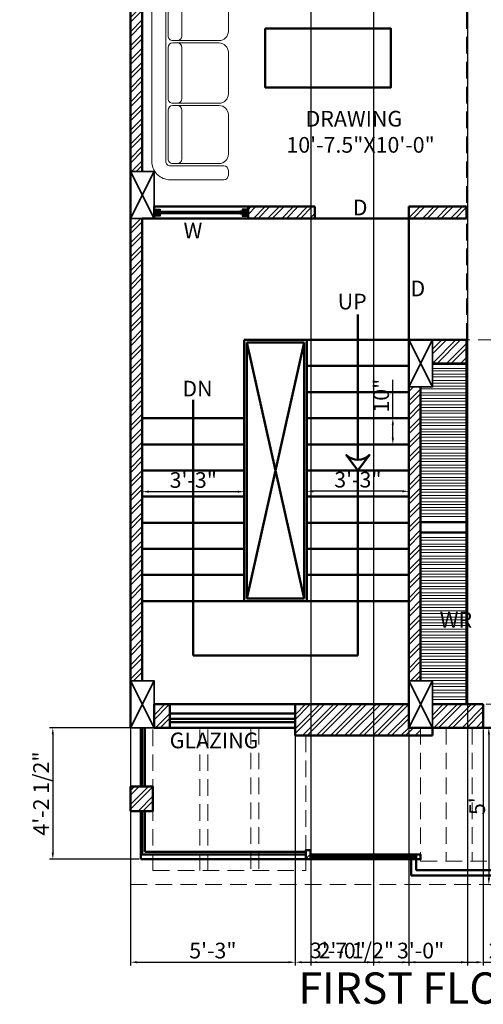
# Model space of a CAD drawing. Units: millimetres. Extents: x 67033 to 68301, y 155969 to 157209.
# Tile 10 of 17: x 67456 to 67633, y 156517 to 156894. Entities that reach past the tile are written whole.
import ezdxf

# ---------------------------------------------------------------- set-up
doc = ezdxf.new("R2010")
doc.units = ezdxf.units.MM
doc.linetypes.add('HIDDEN', pattern=[9.525, 6.35, -3.175])
for name, color, linetype, lineweight in [('A-ANNO-DIMS', 2, 'Continuous', 18), ('A-ANNO-TEXT', 7, 'Continuous', 18), ('A-AREA-IDEN', 3, 'Continuous', 18), ('A-COLS', 3, 'Continuous', 35), ('A-FLOR-OVHD', 1, 'HIDDEN', 18), ('A-FURN', 8, 'Continuous', 18), ('A-GLAZ', 4, 'Continuous', 25), ('A-WALL', 7, 'Continuous', 50), ('A-WALL-PATT', 8, 'Continuous', 13)]:
    doc.layers.add(name, color=color, linetype=linetype, lineweight=lineweight)
doc.styles.get("Standard").update_dxf_attribs({"font": 'arial.ttf'})
doc.dimstyles.new('ISO-25', dxfattribs={"dimtxt": 6, "dimasz": 2.5, "dimexe": 1.25, "dimexo": 0.625, "dimtad": 1, "dimdec": 0, "dimlunit": 3, "dimtxsty": 'Standard', "dimcen": 2.5, "dimadec": 0, "dimazin": 0, "dimtfac": 1, "dimtdec": 0, "dimtmove": 0, "dimatfit": 3, "dimfxl": 1, "dimarcsym": 0})
pattern_1 = [(45, (429.8785, 0), (-2.69407684, 2.69407684), []), (45, (431.6745, 0), (-2.69407684, 2.69407684), [])]

# ---------------------------------------------------------------- blocks, each defined once
blk = doc.blocks.new('A$C2AFA021D')
for p, q in [((0.8, 2.3), (0.2, 2.3)), ((0.85, 2.2), (0.85, 2.25)), ((0.2, 2.15), (0.8, 2.15)), ((0.225, 2.125), (0.275, 2.125)), ((0.75, 2.125), (0.275, 2.125)), ((0, 2.1), (0, 0.2)), ((0.15, 0.2), (0.15, 2.1)), ((0.175, 1.55), (0.175, 2.075)), ((0.325, 2.075), (0.325, 1.55)), ((0.85, 1.6), (0.85, 2.025)), ((0.275, 1.5), (0.225, 1.5)), ((0.275, 1.5), (0.75, 1.5)), ((0.175, 0.875), (0.175, 1.425)), ((0.225, 1.475), (0.275, 1.475)), ((0.75, 1.475), (0.275, 1.475)), ((0.325, 1.425), (0.325, 0.875)), ((0.85, 0.925), (0.85, 1.375)), ((0.175, 0.225), (0.175, 0.75)), ((0.275, 0.825), (0.225, 0.825)), ((0.225, 0.8), (0.275, 0.8)), ((0.275, 0.825), (0.75, 0.825)), ((0.75, 0.8), (0.275, 0.8)), ((0.325, 0.75), (0.325, 0.225)), ((0.975, 0.825), (1.4, 0.825)), ((1.625, 0.825), (2.075, 0.825)), ((2.3, 0.825), (2.725, 0.825)), ((2.85, 0.2), (2.85, 0.775)), ((2.9, 0.825), (2.95, 0.825)), ((3, 0.775), (3, 0.2)), ((0.85, 0.275), (0.85, 0.7)), ((0.875, 0.275), (0.875, 0.725)), ((1.5, 0.725), (1.5, 0.275)), ((1.525, 0.275), (1.525, 0.725)), ((2.175, 0.725), (2.175, 0.275)), ((2.2, 0.275), (2.2, 0.725)), ((2.825, 0.725), (2.825, 0.275)), ((1.45, 0.325), (0.925, 0.325)), ((2.125, 0.325), (1.575, 0.325)), ((2.775, 0.325), (2.25, 0.325)), ((0.875, 0.275), (0.875, 0.225)), ((1.5, 0.225), (1.5, 0.275)), ((1.525, 0.275), (1.525, 0.225)), ((2.175, 0.225), (2.175, 0.275)), ((2.2, 0.275), (2.2, 0.225)), ((2.825, 0.225), (2.825, 0.275)), ((0.8, 0.15), (0.2, 0.15)), ((0.275, 0.175), (0.225, 0.175)), ((0.275, 0.175), (0.75, 0.175)), ((0.925, 0.175), (1.45, 0.175)), ((0.925, 0.15), (2.8, 0.15)), ((1.575, 0.175), (2.125, 0.175)), ((2.25, 0.175), (2.775, 0.175)), ((0.85, 0), (0.85, 0.1)), ((0.875, 0.1), (0.875, 0)), ((0.2, 0), (0.85, 0)), ((2.8, 0), (0.875, 0))]:
    blk.add_line(p, q)
for centre, radius, start, end in [((0.2, 2.1), 0.2, 90, 180), ((0.8, 2.25), 0.05, 0, 90), ((0.2, 2.1), 0.05, 90, 180), ((0.225, 2.075), 0.05, 90, 180), ((0.275, 2.075), 0.05, 0, 90), ((0.75, 2.025), 0.1, 0, 90), ((0.8, 2.2), 0.05, 270, 0), ((0.75, 1.6), 0.1, 270, 0), ((0.225, 1.55), 0.05, 180, 270), ((0.275, 1.55), 0.05, 270, 0), ((0.225, 1.425), 0.05, 90, 180), ((0.275, 1.425), 0.05, 0, 90), ((0.75, 1.375), 0.1, 360, 90), ((0.225, 0.875), 0.05, 180, 270), ((0.275, 0.875), 0.05, 270, 0), ((0.75, 0.925), 0.1, 270, 0), ((0.225, 0.75), 0.05, 90, 180), ((0.275, 0.75), 0.05, 0, 90), ((0.75, 0.7), 0.1, 0, 90), ((0.975, 0.725), 0.1, 90, 180), ((1.4, 0.725), 0.1, 0, 90), ((1.625, 0.725), 0.1, 90, 180), ((2.075, 0.725), 0.1, 0, 90), ((2.3, 0.725), 0.1, 90, 180), ((2.725, 0.725), 0.1, 0, 90), ((2.9, 0.775), 0.05, 90, 180), ((2.95, 0.775), 0.05, 0, 90), ((0.925, 0.275), 0.05, 90, 180), ((1.45, 0.275), 0.05, 360, 90), ((1.575, 0.275), 0.05, 90, 180), ((2.125, 0.275), 0.05, 360, 90), ((2.25, 0.275), 0.05, 90, 180), ((2.775, 0.275), 0.05, 360, 90), ((0.225, 0.225), 0.05, 180, 270), ((0.275, 0.225), 0.05, 270, 0), ((0.75, 0.275), 0.1, 270, 0), ((0.925, 0.225), 0.05, 180, 270), ((1.45, 0.225), 0.05, 270, 0), ((1.575, 0.225), 0.05, 180, 270), ((2.125, 0.225), 0.05, 270, 0), ((2.25, 0.225), 0.05, 180, 270), ((2.775, 0.225), 0.05, 270, 0), ((0.2, 0.2), 0.2, 180, 270), ((0.2, 0.2), 0.05, 180, 270), ((0.8, 0.1), 0.05, 0, 90), ((0.925, 0.1), 0.05, 90, 180), ((2.8, 0.2), 0.2, 270, 0), ((2.8, 0.2), 0.05, 270, 0)]:
    blk.add_arc(centre, radius, start, end)
blk = doc.blocks.new('*D35')
at = {"layer": 'A-ANNO-DIMS', "color": 0, "lineweight": -2, "transparency": 16777216}
for p, q in [((67565.82, 156713.06), (67565.82, 156711.77)), ((67602.32, 156713.02), (67568.32, 156713.02)), ((67604.82, 156713.06), (67604.82, 156711.77))]:
    blk.add_line(p, q, dxfattribs=at)
at = {"layer": 'A-ANNO-DIMS', "color": 0, "transparency": 16777216}
for points in [[(67568.32, 156713.44), (67568.32, 156712.61), (67565.82, 156713.02)], [(67602.32, 156713.44), (67602.32, 156712.61), (67604.82, 156713.02)]]:
    blk.add_solid(points, dxfattribs=at)
at = {"layer": 'Defpoints', "color": 0, "transparency": 16777216}
for p in [(67565.82, 156713.68), (67565.82, 156713.02), (67604.82, 156713.68)]:
    blk.add_point(p, dxfattribs=at)
at = {"layer": 'A-ANNO-DIMS', "color": 0, "transparency": 16777216, "insert": (67585.32, 156716.71), "char_height": 6, "attachment_point": 5}
blk.add_mtext('3\'-3"', dxfattribs=at)
blk = doc.blocks.new('*D36')
at = {"layer": 'A-ANNO-DIMS', "color": 0, "lineweight": -2, "transparency": 16777216}
for p, q in [((67539.32, 156712.88), (67505.32, 156712.88)), ((67502.82, 156712.4), (67502.82, 156711.63)), ((67541.82, 156712.4), (67541.82, 156711.63))]:
    blk.add_line(p, q, dxfattribs=at)
at = {"layer": 'A-ANNO-DIMS', "color": 0, "transparency": 16777216}
for points in [[(67505.32, 156713.29), (67505.32, 156712.46), (67502.82, 156712.88)], [(67539.32, 156713.29), (67539.32, 156712.46), (67541.82, 156712.88)]]:
    blk.add_solid(points, dxfattribs=at)
at = {"layer": 'Defpoints', "color": 0, "transparency": 16777216}
for p in [(67502.82, 156713.02), (67502.82, 156712.88), (67541.82, 156713.02)]:
    blk.add_point(p, dxfattribs=at)
at = {"layer": 'A-ANNO-DIMS', "color": 0, "transparency": 16777216, "insert": (67522.32, 156716.57), "char_height": 6, "attachment_point": 5}
blk.add_mtext('3\'-3"', dxfattribs=at)
blk = doc.blocks.new('*D33')
at = {"layer": 'A-ANNO-DIMS', "color": 0, "lineweight": -2, "transparency": 16777216}
for p, q in [((67598.69, 156740.99), (67598.69, 156755.74)), ((67599.31, 156740.99), (67599.94, 156740.99)), ((67598.69, 156733.49), (67598.69, 156738.49)), ((67599.31, 156730.99), (67599.94, 156730.99))]:
    blk.add_line(p, q, dxfattribs=at)
at = {"layer": 'A-ANNO-DIMS', "color": 0, "transparency": 16777216}
for points in [[(67598.27, 156738.49), (67599.11, 156738.49), (67598.69, 156740.99)], [(67598.27, 156733.49), (67599.11, 156733.49), (67598.69, 156730.99)]]:
    blk.add_solid(points, dxfattribs=at)
at = {"layer": 'Defpoints', "color": 0, "transparency": 16777216}
for p in [(67598.69, 156740.99), (67598.69, 156740.99), (67598.69, 156730.99)]:
    blk.add_point(p, dxfattribs=at)
at = {"layer": 'A-ANNO-DIMS', "color": 0, "transparency": 16777216, "insert": (67595, 156749.62), "char_height": 6, "attachment_point": 5, "rotation": 90}
blk.add_mtext('10"', dxfattribs=at)
blk = doc.blocks.new('*D37')
at = {"layer": 'A-ANNO-DIMS', "color": 0, "lineweight": -2, "transparency": 16777216}
for p, q in [((67636.06, 156622.49), (67636.68, 156622.49)), ((67635.43, 156619.99), (67635.43, 156564.99)), ((67636.06, 156562.49), (67636.68, 156562.49))]:
    blk.add_line(p, q, dxfattribs=at)
at = {"layer": 'A-ANNO-DIMS', "color": 0, "transparency": 16777216}
for points in [[(67635.02, 156619.99), (67635.85, 156619.99), (67635.43, 156622.49)], [(67635.02, 156564.99), (67635.85, 156564.99), (67635.43, 156562.49)]]:
    blk.add_solid(points, dxfattribs=at)
at = {"layer": 'Defpoints', "color": 0, "transparency": 16777216}
for p in [(67635.43, 156622.49), (67635.43, 156562.49), (67635.43, 156562.49)]:
    blk.add_point(p, dxfattribs=at)
at = {"layer": 'A-ANNO-DIMS', "color": 0, "transparency": 16777216, "insert": (67631.76, 156592.49), "char_height": 6, "attachment_point": 5, "rotation": 90}
blk.add_mtext("5'", dxfattribs=at)
blk = doc.blocks.new('WIN-900')
for p, q in [((3.67, 3.22), (33.2, 3.22)), ((3.67, 2.74), (33.2, 2.74)), ((33.2, 2.27), (3.67, 2.27))]:
    blk.add_line(p, q)
blk.add_lwpolyline([(0.44, 4.99), (36.44, 4.99), (36.44, 0.49), (0.44, 0.49)], close=True)
for points in [[(0.44, 4.09), (2.73, 4.09), (2.73, 3.22), (3.67, 3.22), (3.67, 2.27), (2.73, 2.27), (2.73, 1.4), (0.44, 1.4)], [(36.44, 4.09), (34.14, 4.09), (34.14, 3.22), (33.2, 3.22), (33.2, 2.27), (34.14, 2.27), (34.14, 1.4), (36.44, 1.4)]]:
    blk.add_lwpolyline(points)
blk = doc.blocks.new('COLUMN-230x460')
for p, q in [((0.44, 17.99), (9.44, -0.01)), ((9.44, 17.99), (0.44, -0.01))]:
    blk.add_line(p, q)
blk.add_lwpolyline([(0.44, 17.99), (9.44, 17.99), (9.44, -0.01), (0.44, -0.01)], close=True)
blk = doc.blocks.new('*D96')
at = {"layer": 'A-ANNO-DIMS', "color": 0, "lineweight": -2, "transparency": 16777216}
for p, q in [((67567.32, 157082.37), (67567.32, 156531.49)), ((67591.32, 157082.37), (67591.32, 156531.49)), ((67569.82, 156532.74), (67588.82, 156532.74))]:
    blk.add_line(p, q, dxfattribs=at)
at = {"layer": 'A-ANNO-DIMS', "color": 0, "transparency": 16777216}
for points in [[(67569.82, 156533.16), (67569.82, 156532.33), (67567.32, 156532.74)], [(67588.82, 156533.16), (67588.82, 156532.33), (67591.32, 156532.74)]]:
    blk.add_solid(points, dxfattribs=at)
at = {"layer": 'Defpoints', "color": 0, "transparency": 16777216}
for p in [(67567.32, 157082.99), (67591.32, 157082.99), (67591.32, 156532.74)]:
    blk.add_point(p, dxfattribs=at)
at = {"layer": 'A-ANNO-DIMS', "color": 0, "transparency": 16777216, "insert": (67579.32, 156536.43), "char_height": 6, "attachment_point": 5}
blk.add_mtext('2\'-0"', dxfattribs=at)
blk = doc.blocks.new('*D97')
at = {"layer": 'A-ANNO-DIMS', "color": 0, "lineweight": -2, "transparency": 16777216}
for p, q in [((67591.32, 157082.37), (67591.32, 156531.49)), ((67627.32, 157082.37), (67627.32, 156531.49)), ((67593.82, 156532.74), (67624.82, 156532.74))]:
    blk.add_line(p, q, dxfattribs=at)
at = {"layer": 'A-ANNO-DIMS', "color": 0, "transparency": 16777216}
for points in [[(67593.82, 156533.16), (67593.82, 156532.33), (67591.32, 156532.74)], [(67624.82, 156533.16), (67624.82, 156532.33), (67627.32, 156532.74)]]:
    blk.add_solid(points, dxfattribs=at)
at = {"layer": 'Defpoints', "color": 0, "transparency": 16777216}
for p in [(67591.32, 157082.99), (67627.32, 157082.99), (67627.32, 156532.74)]:
    blk.add_point(p, dxfattribs=at)
at = {"layer": 'A-ANNO-DIMS', "color": 0, "transparency": 16777216, "insert": (67609.32, 156536.43), "char_height": 6, "attachment_point": 5}
blk.add_mtext('3\'-0"', dxfattribs=at)
blk = doc.blocks.new('*D103')
at = {"layer": 'A-ANNO-DIMS', "color": 0, "lineweight": -2, "transparency": 16777216}
for p, q in [((67498.32, 156621.85), (67498.32, 156531.49)), ((67561.32, 156621.85), (67561.32, 156531.49)), ((67500.82, 156532.74), (67558.82, 156532.74))]:
    blk.add_line(p, q, dxfattribs=at)
at = {"layer": 'A-ANNO-DIMS', "color": 0, "transparency": 16777216}
for points in [[(67500.82, 156533.16), (67500.82, 156532.33), (67498.32, 156532.74)], [(67558.82, 156533.16), (67558.82, 156532.33), (67561.32, 156532.74)]]:
    blk.add_solid(points, dxfattribs=at)
at = {"layer": 'Defpoints', "color": 0, "transparency": 16777216}
for p in [(67498.32, 156622.48), (67561.32, 156622.48), (67561.32, 156532.74)]:
    blk.add_point(p, dxfattribs=at)
at = {"layer": 'A-ANNO-DIMS', "color": 0, "transparency": 16777216, "insert": (67529.82, 156536.43), "char_height": 6, "attachment_point": 5}
blk.add_mtext('5\'-3"', dxfattribs=at)
blk = doc.blocks.new('*D104')
at = {"layer": 'A-ANNO-DIMS', "color": 0, "lineweight": -2, "transparency": 16777216}
for p, q in [((67561.32, 156621.85), (67561.32, 156531.49)), ((67604.81, 156621.86), (67604.81, 156531.49)), ((67563.82, 156532.74), (67602.31, 156532.74))]:
    blk.add_line(p, q, dxfattribs=at)
at = {"layer": 'A-ANNO-DIMS', "color": 0, "transparency": 16777216}
for points in [[(67563.82, 156533.16), (67563.82, 156532.33), (67561.32, 156532.74)], [(67602.31, 156533.16), (67602.31, 156532.33), (67604.81, 156532.74)]]:
    blk.add_solid(points, dxfattribs=at)
at = {"layer": 'Defpoints', "color": 0, "transparency": 16777216}
for p in [(67561.32, 156622.48), (67604.81, 156622.48), (67604.81, 156532.74)]:
    blk.add_point(p, dxfattribs=at)
at = {"layer": 'A-ANNO-DIMS', "color": 0, "transparency": 16777216, "insert": (67583.06, 156536.47), "char_height": 6, "attachment_point": 5}
blk.add_mtext('3\'-7 1/2"', dxfattribs=at)
blk = doc.blocks.new('*D105')
at = {"layer": 'A-ANNO-DIMS', "color": 0, "lineweight": -2, "transparency": 16777216}
for p, q in [((67604.81, 156621.86), (67604.81, 156531.49)), ((67633.32, 156621.87), (67633.32, 156531.49)), ((67607.31, 156532.74), (67630.82, 156532.74)), ((67633.32, 156532.74), (67667.1, 156532.74))]:
    blk.add_line(p, q, dxfattribs=at)
at = {"layer": 'A-ANNO-DIMS', "color": 0, "transparency": 16777216}
for points in [[(67607.31, 156533.16), (67607.31, 156532.33), (67604.81, 156532.74)], [(67630.82, 156533.16), (67630.82, 156532.33), (67633.32, 156532.74)]]:
    blk.add_solid(points, dxfattribs=at)
at = {"layer": 'Defpoints', "color": 0, "transparency": 16777216}
for p in [(67604.81, 156622.48), (67633.32, 156622.49), (67633.32, 156532.74)]:
    blk.add_point(p, dxfattribs=at)
at = {"layer": 'A-ANNO-DIMS', "color": 0, "transparency": 16777216, "insert": (67651.46, 156536.47), "char_height": 6, "attachment_point": 5}
blk.add_mtext('2\'-4 1/2"', dxfattribs=at)
blk = doc.blocks.new('*D112')
at = {"layer": 'A-ANNO-DIMS', "color": 0, "lineweight": -2, "transparency": 16777216}
for p, q in [((67601.44, 157144.49), (67868.32, 157144.49)), ((67867.07, 157141.99), (67867.07, 156564.99)), ((67768.94, 156562.49), (67868.32, 156562.49))]:
    blk.add_line(p, q, dxfattribs=at)
at = {"layer": 'A-ANNO-DIMS', "color": 0, "transparency": 16777216}
for points in [[(67866.65, 157141.99), (67867.48, 157141.99), (67867.07, 157144.49)], [(67866.65, 156564.99), (67867.48, 156564.99), (67867.07, 156562.49)]]:
    blk.add_solid(points, dxfattribs=at)
at = {"layer": 'Defpoints', "color": 0, "transparency": 16777216}
for p in [(67600.82, 157144.49), (67768.32, 156562.49), (67867.07, 156562.49)]:
    blk.add_point(p, dxfattribs=at)
at = {"layer": 'A-ANNO-DIMS', "color": 0, "transparency": 16777216, "insert": (67863.38, 156853.49), "char_height": 6, "attachment_point": 5, "rotation": 90}
blk.add_mtext('48\'-6"', dxfattribs=at)
blk = doc.blocks.new('*D113')
at = {"layer": 'A-ANNO-DIMS', "color": 0, "lineweight": -2, "transparency": 16777216}
for p, q in [((67501.61, 156622.48), (67467.32, 156622.48)), ((67468.57, 156619.98), (67468.57, 156574.65)), ((67501.61, 156572.15), (67467.32, 156572.15))]:
    blk.add_line(p, q, dxfattribs=at)
at = {"layer": 'A-ANNO-DIMS', "color": 0, "transparency": 16777216}
for points in [[(67468.15, 156619.98), (67468.98, 156619.98), (67468.57, 156622.48)], [(67468.15, 156574.65), (67468.98, 156574.65), (67468.57, 156572.15)]]:
    blk.add_solid(points, dxfattribs=at)
at = {"layer": 'Defpoints', "color": 0, "transparency": 16777216}
for p in [(67502.23, 156622.48), (67468.57, 156572.15), (67502.23, 156572.15)]:
    blk.add_point(p, dxfattribs=at)
at = {"layer": 'A-ANNO-DIMS', "color": 0, "transparency": 16777216, "insert": (67464.84, 156597.31), "char_height": 6, "attachment_point": 5, "rotation": 90}
blk.add_mtext('4\'-2 1/2"', dxfattribs=at)

msp = doc.modelspace()

# ---------------------------------------------------------------- hatches: boundary and pattern name
at = {"layer": 'A-GLAZ'}
h = msp.add_hatch(color=256, dxfattribs=at)
h.dxf.hatch_style = 1
h.paths.add_polyline_path([(67510.55, 156820.22), (67509.61, 156820.22), (67509.61, 156821.09), (67507.32, 156821.09), (67507.32, 156818.4), (67509.61, 156818.4), (67509.61, 156819.27), (67510.55, 156819.27)])
h = msp.add_hatch(color=256, dxfattribs=at)
h.dxf.hatch_style = 1
h.paths.add_polyline_path([(67543.32, 156821.09), (67541.02, 156821.09), (67541.02, 156820.22), (67540.08, 156820.22), (67540.08, 156819.27), (67541.02, 156819.27), (67541.02, 156818.4), (67543.32, 156818.4)])
at = {"layer": 'A-WALL-PATT'}
h = msp.add_hatch(dxfattribs=at)
h.set_pattern_fill('ANSI32', color=256, scale=0.4)
h.set_pattern_definition(pattern_1)
h.paths.add_polyline_path([(67502.82, 157064.99), (67498.32, 157064.99), (67498.32, 156835.49), (67502.82, 156835.49), (67502.82, 156941.99), (67626.86, 156941.99), (67626.86, 156946.49), (67502.82, 156946.49)])
h = msp.add_hatch(dxfattribs=at)
h.set_pattern_fill('ANSI32', color=256, scale=0.4)
h.set_pattern_definition(pattern_1)
h.paths.add_polyline_path([(67568.82, 156821.99), (67543.32, 156821.99), (67543.32, 156817.49), (67568.82, 156817.49)])
h = msp.add_hatch(dxfattribs=at)
h.set_pattern_fill('ANSI32', color=256, scale=0.4)
h.set_pattern_definition(pattern_1)
h.paths.add_polyline_path([(67626.86, 156821.99), (67604.82, 156821.99), (67604.82, 156817.49), (67626.86, 156817.49)])
h = msp.add_hatch(dxfattribs=at)
h.set_pattern_fill('ANSI32', color=256, scale=0.4)
h.set_pattern_definition(pattern_1)
h.paths.add_polyline_path([(67502.82, 156817.49), (67498.32, 156817.49), (67498.32, 156640.48), (67502.82, 156640.48)])
h = msp.add_hatch(dxfattribs=at)
h.set_pattern_fill('ANSI32', color=256, scale=0.4)
h.set_pattern_definition(pattern_1)
h.paths.add_polyline_path([(67626.86, 156770.99), (67613.82, 156770.99), (67613.82, 156761.99), (67626.86, 156761.99)])
h = msp.add_hatch(dxfattribs=at)
h.set_pattern_fill('ANSI32', color=256, scale=0.4)
h.set_pattern_definition(pattern_1)
h.paths.add_polyline_path([(67609.32, 156752.99), (67604.82, 156752.99), (67604.82, 156640.48), (67609.32, 156640.48)])
h = msp.add_hatch(dxfattribs=at)
h.set_pattern_fill('ANSI32', color=256, scale=0.4)
h.paths.add_polyline_path([(67513.32, 156631.49), (67507.32, 156631.49), (67507.32, 156622.48), (67513.32, 156622.48)])
h = msp.add_hatch(dxfattribs=at)
h.set_pattern_fill('ANSI32', color=256, scale=0.4)
h.paths.add_polyline_path([(67604.82, 156631.49), (67561.32, 156631.49), (67561.32, 156622.48), (67561.32, 156619.48), (67609.32, 156619.48), (67609.32, 156622.48), (67604.81, 156622.48), (67604.82, 156622.49)])
h = msp.add_hatch(dxfattribs=at)
h.set_pattern_fill('ANSI32', color=256, scale=0.4)
h.set_pattern_definition(pattern_1)
h.paths.add_polyline_path([(67633.32, 156631.49), (67613.82, 156631.49), (67613.82, 156622.49), (67633.32, 156622.49)])
h = msp.add_hatch(dxfattribs=at)
h.set_pattern_fill('ANSI32', color=256, scale=0.4)
h.set_pattern_definition([(45, (323.3785, 23.292), (-2.69407684, 2.69407684), []), (45, (325.1745, 23.292), (-2.69407684, 2.69407684), [])])
h.paths.add_polyline_path([(67506.87, 156600.01), (67498.32, 156600.01), (67498.32, 156590.61), (67506.87, 156590.61)])
h = msp.add_hatch(dxfattribs=at)
h.set_pattern_fill('ANSI32', color=256, scale=0.4)
h.paths.add_polyline_path([(67567.18, 156575.67), (67565.37, 156575.67), (67565.37, 156572.15), (67567.18, 156572.15)])

# ---------------------------------------------------------------- linework, layer by layer
at = {"layer": 'A-FLOR-OVHD'}
for p, q in [((67626.86, 156905.99), (67626.86, 156821.99)), ((67626.86, 156770.99), (67626.86, 156817.49)), ((67666.32, 156770.99), (67626.86, 156770.99)), ((67669.32, 156631.49), (67633.32, 156631.49)), ((67498.32, 156622.48), (67498.32, 156562.49)), ((67506.87, 156567.85), (67506.87, 156622.48)), ((67524.87, 156567.85), (67524.87, 156622.48)), ((67527.87, 156567.85), (67527.87, 156622.48)), ((67544.37, 156622.48), (67544.37, 156567.85)), ((67547.37, 156622.49), (67547.37, 156567.85)), ((67609.32, 156622.48), (67609.32, 156571.49)), ((67619.07, 156622.49), (67619.07, 156571.49)), ((67629.07, 156622.49), (67629.07, 156571.49)), ((67565.37, 156619.48), (67565.37, 156567.85)), ((67609.32, 156571.49), (67768.32, 156571.49)), ((67506.87, 156567.85), (67565.37, 156567.85)), ((67498.32, 156562.49), (67732.32, 156562.49))]:
    msp.add_line(p, q, dxfattribs=at)
at = {"layer": 'A-FURN'}
for p, q in [((67613.82, 156761.54), (67626.86, 156761.54)), ((67613.82, 156760.09), (67626.86, 156760.09)), ((67613.82, 156759.09), (67626.86, 156759.09)), ((67613.82, 156757.87), (67626.86, 156757.87)), ((67613.82, 156756.87), (67626.86, 156756.87)), ((67613.82, 156755.43), (67626.86, 156755.43)), ((67613.82, 156754.43), (67626.86, 156754.43)), ((67609.32, 156752.21), (67626.86, 156752.21)), ((67609.32, 156750.77), (67626.86, 156750.77)), ((67613.71, 156753.21), (67626.86, 156753.21)), ((67609.32, 156749.77), (67626.86, 156749.77)), ((67609.32, 156748.55), (67626.86, 156748.55)), ((67609.32, 156747.55), (67626.86, 156747.55)), ((67609.32, 156746.1), (67626.86, 156746.1)), ((67609.32, 156745.1), (67626.86, 156745.1)), ((67609.32, 156743.88), (67626.86, 156743.88)), ((67609.32, 156742.88), (67626.86, 156742.88)), ((67609.32, 156741.44), (67626.86, 156741.44)), ((67609.32, 156740.44), (67626.86, 156740.44)), ((67609.32, 156739.22), (67626.86, 156739.22)), ((67609.32, 156738.22), (67626.86, 156738.22)), ((67609.32, 156736.78), (67626.86, 156736.78)), ((67609.32, 156735.78), (67626.86, 156735.78)), ((67609.32, 156734.76), (67626.86, 156734.76)), ((67609.32, 156733.76), (67626.86, 156733.76)), ((67609.32, 156732.32), (67626.86, 156732.32)), ((67609.32, 156731.32), (67626.86, 156731.32)), ((67609.32, 156730.1), (67626.86, 156730.1)), ((67609.32, 156729.1), (67626.86, 156729.1)), ((67609.32, 156727.66), (67626.86, 156727.66)), ((67609.32, 156726.66), (67626.86, 156726.66)), ((67609.32, 156725.44), (67626.86, 156725.44)), ((67609.32, 156724.44), (67626.86, 156724.44)), ((67609.32, 156722.99), (67626.86, 156722.99)), ((67609.32, 156721.99), (67626.86, 156721.99)), ((67609.32, 156720.77), (67626.86, 156720.77)), ((67609.32, 156719.77), (67626.86, 156719.77)), ((67609.32, 156718.33), (67626.86, 156718.33)), ((67609.32, 156717.33), (67626.86, 156717.33)), ((67609.32, 156716.11), (67626.86, 156716.11)), ((67609.32, 156715.11), (67626.86, 156715.11)), ((67609.32, 156713.67), (67626.86, 156713.67)), ((67609.32, 156712.67), (67626.86, 156712.67)), ((67609.32, 156711.45), (67626.86, 156711.45)), ((67609.32, 156710.45), (67626.86, 156710.45)), ((67609.32, 156709.01), (67626.86, 156709.01)), ((67609.32, 156708.01), (67626.86, 156708.01)), ((67609.32, 156706.79), (67626.86, 156706.79)), ((67609.32, 156705.79), (67626.86, 156705.79)), ((67609.32, 156704.34), (67626.86, 156704.34)), ((67609.32, 156703.34), (67626.86, 156703.34)), ((67609.32, 156695.28), (67626.86, 156695.28)), ((67609.32, 156694.28), (67626.86, 156694.28)), ((67609.32, 156692.84), (67626.86, 156692.84)), ((67609.32, 156691.84), (67626.86, 156691.84)), ((67609.32, 156690.62), (67626.86, 156690.62)), ((67609.32, 156689.62), (67626.86, 156689.62)), ((67609.32, 156688.17), (67626.86, 156688.17)), ((67609.32, 156687.17), (67626.86, 156687.17)), ((67609.32, 156685.95), (67626.86, 156685.95)), ((67609.32, 156684.95), (67626.86, 156684.95)), ((67609.32, 156683.51), (67626.86, 156683.51)), ((67609.32, 156682.51), (67626.86, 156682.51)), ((67609.32, 156681.29), (67626.86, 156681.29)), ((67609.32, 156680.29), (67626.86, 156680.29)), ((67609.32, 156678.85), (67626.86, 156678.85)), ((67609.32, 156677.85), (67626.86, 156677.85)), ((67609.32, 156676.63), (67626.86, 156676.63)), ((67609.32, 156675.63), (67626.86, 156675.63)), ((67609.32, 156674.19), (67626.86, 156674.19)), ((67609.32, 156673.19), (67626.86, 156673.19)), ((67609.32, 156671.97), (67626.86, 156671.97)), ((67609.32, 156670.97), (67626.86, 156670.97)), ((67609.32, 156669.52), (67626.86, 156669.52)), ((67609.32, 156668.52), (67626.86, 156668.52)), ((67609.32, 156667.3), (67626.86, 156667.3)), ((67609.32, 156666.3), (67626.86, 156666.3)), ((67609.32, 156664.86), (67626.86, 156664.86)), ((67609.32, 156663.86), (67626.86, 156663.86)), ((67609.32, 156662.64), (67626.86, 156662.64)), ((67609.32, 156661.64), (67626.86, 156661.64)), ((67609.32, 156660.2), (67626.86, 156660.2)), ((67609.32, 156659.2), (67626.86, 156659.2)), ((67609.32, 156657.98), (67626.86, 156657.98)), ((67609.32, 156656.98), (67626.86, 156656.98)), ((67609.32, 156655.53), (67626.86, 156655.53)), ((67609.32, 156654.53), (67626.86, 156654.53)), ((67609.32, 156653.31), (67626.86, 156653.31)), ((67609.32, 156652.31), (67626.86, 156652.31)), ((67609.32, 156650.87), (67626.86, 156650.87)), ((67609.32, 156649.87), (67626.86, 156649.87)), ((67609.32, 156648.65), (67626.86, 156648.65)), ((67609.32, 156647.65), (67626.86, 156647.65)), ((67609.32, 156646.21), (67626.86, 156646.21)), ((67609.32, 156645.21), (67626.86, 156645.21)), ((67609.32, 156643.99), (67626.86, 156643.99)), ((67609.32, 156642.99), (67626.86, 156642.99)), ((67609.32, 156641.55), (67626.86, 156641.55)), ((67609.32, 156640.55), (67626.86, 156640.55)), ((67613.82, 156639.33), (67626.86, 156639.33)), ((67613.82, 156638.33), (67626.86, 156638.33)), ((67613.82, 156636.89), (67626.86, 156636.89)), ((67613.82, 156635.89), (67626.86, 156635.89)), ((67613.82, 156634.35), (67626.86, 156634.35)), ((67613.82, 156633.35), (67626.86, 156633.35))]:
    msp.add_line(p, q, dxfattribs=at)
at = {"layer": 'A-WALL'}
for p, q in [((67498.32, 157136.99), (67498.32, 156622.48)), ((67502.82, 156941.99), (67502.82, 156835.49)), ((67507.32, 156821.99), (67568.82, 156821.99)), ((67507.32, 156821.99), (67507.32, 156817.49)), ((67543.32, 156821.99), (67543.32, 156817.49)), ((67568.82, 156821.99), (67568.82, 156817.49)), ((67604.82, 156821.99), (67604.82, 156622.49)), ((67604.82, 156821.99), (67626.86, 156821.99)), ((67626.86, 156821.99), (67626.86, 156817.49)), ((67502.82, 156817.49), (67502.82, 156640.48)), ((67502.82, 156817.49), (67568.82, 156817.49)), ((67604.82, 156817.49), (67568.82, 156817.49)), ((67604.82, 156817.49), (67626.86, 156817.49)), ((67585.32, 156725.08), (67585.32, 156780.67)), ((67541.82, 156770.99), (67541.82, 156670.99)), ((67541.82, 156770.99), (67604.82, 156770.99)), ((67542.82, 156769.99), (67542.82, 156671.99)), ((67542.82, 156769.99), (67564.82, 156769.99)), ((67542.82, 156769.99), (67564.82, 156671.99)), ((67542.82, 156671.99), (67564.82, 156769.99)), ((67564.82, 156769.99), (67564.82, 156671.99)), ((67565.82, 156770.99), (67565.82, 156670.99)), ((67604.82, 156770.99), (67626.86, 156770.99)), ((67626.86, 156770.99), (67626.86, 156631.49)), ((67613.82, 156761.99), (67626.86, 156761.99)), ((67565.82, 156760.99), (67604.82, 156760.99)), ((67565.82, 156750.99), (67604.82, 156750.99)), ((67609.32, 156752.99), (67609.32, 156640.48)), ((67522.32, 156747.98), (67522.32, 156650.15)), ((67502.82, 156740.99), (67541.82, 156740.99)), ((67565.82, 156740.99), (67604.82, 156740.99)), ((67502.82, 156730.99), (67541.82, 156730.99)), ((67565.82, 156730.99), (67604.82, 156730.99)), ((67502.82, 156720.99), (67541.82, 156720.99)), ((67565.82, 156720.99), (67604.82, 156720.99)), ((67585.32, 156720.99), (67585.32, 156650.15)), ((67502.82, 156710.99), (67541.82, 156710.99)), ((67565.82, 156710.99), (67604.82, 156710.99)), ((67502.82, 156700.99), (67541.82, 156700.99)), ((67565.82, 156700.99), (67604.82, 156700.99)), ((67626.86, 156701.24), (67609.32, 156701.24)), ((67626.86, 156697.24), (67609.32, 156697.24)), ((67502.82, 156690.99), (67541.82, 156690.99)), ((67565.82, 156690.99), (67604.82, 156690.99)), ((67502.82, 156680.99), (67541.82, 156680.99)), ((67565.82, 156680.99), (67604.82, 156680.99)), ((67542.82, 156671.99), (67564.82, 156671.99)), ((67502.82, 156670.99), (67565.82, 156670.99)), ((67565.82, 156670.99), (67604.82, 156670.99)), ((67522.32, 156650.15), (67585.32, 156650.15)), ((67604.82, 156631.49), (67507.32, 156631.49)), ((67507.32, 156631.48), (67507.32, 156622.48)), ((67513.32, 156631.48), (67513.32, 156622.48)), ((67561.32, 156631.48), (67561.32, 156622.48)), ((67613.82, 156631.49), (67633.32, 156631.49)), ((67633.32, 156631.49), (67633.32, 156622.49)), ((67513.32, 156627.98), (67561.32, 156627.98)), ((67513.32, 156625.98), (67561.32, 156625.98)), ((67502.23, 156600.01), (67502.23, 156622.48)), ((67502.82, 156622.48), (67502.82, 156600.01)), ((67503.82, 156622.48), (67503.82, 156600.01)), ((67507.32, 156622.48), (67561.32, 156622.49)), ((67513.32, 156624.61), (67561.32, 156624.61)), ((67561.32, 156622.48), (67561.32, 156619.48)), ((67604.82, 156622.49), (67633.32, 156622.49)), ((67613.82, 156619.48), (67613.82, 156622.49)), ((67633.32, 156622.49), (67669.32, 156622.49)), ((67561.32, 156619.48), (67613.82, 156619.48)), ((67502.23, 156572.15), (67502.23, 156590.61)), ((67502.82, 156590.61), (67502.82, 156573.95)), ((67503.82, 156590.61), (67503.82, 156574.95)), ((67565.37, 156573.95), (67502.82, 156573.95)), ((67565.37, 156574.95), (67503.82, 156574.95)), ((67607.66, 156573.95), (67567.18, 156573.95)), ((67605.66, 156572.15), (67502.23, 156572.15)), ((67607.66, 156573.05), (67567.18, 156573.05)), ((67605.66, 156572.15), (67605.66, 156565.99)), ((67607.66, 156572.15), (67605.66, 156572.15)), ((67607.66, 156572.15), (67607.66, 156567.99)), ((67723.32, 156565.99), (67605.66, 156565.99)), ((67723.32, 156567.99), (67607.66, 156567.99))]:
    msp.add_line(p, q, dxfattribs=at)
for points in [[(67549.85, 156890.16), (67597.94, 156890.16), (67597.94, 156867.66), (67549.85, 156867.66)], [(67498.32, 156590.61), (67506.87, 156590.61), (67506.87, 156600.01), (67498.32, 156600.01)], [(67565.37, 156572.15), (67567.18, 156572.15), (67567.18, 156575.67), (67565.37, 156575.67)], [(67607.66, 156572.15), (67609.32, 156572.15), (67609.32, 156573.95), (67607.66, 156573.95)]]:
    msp.add_lwpolyline(points, close=True, dxfattribs=at)
msp.add_lwpolyline([(67585.32, 156720.99), (67580.86, 156726.93, 0.414166), (67589.77, 156726.93)], format="xyb", close=True, dxfattribs=at)

# ---------------------------------------------------------------- block references
at = {"layer": 'A-COLS'}
for p in [(67497.88, 156817.5), (67604.38, 156753), (67497.88, 156622.49)]:
    msp.add_blockref('COLUMN-230x460', p, dxfattribs=at)
at = {"layer": 'A-COLS', "extrusion": (0, 0, -1), "zscale": -1, "rotation": 180.0076170408173}
msp.add_blockref('COLUMN-230x460', (-67604.38, 156640.48), dxfattribs=at)
at = {"layer": 'A-FURN', "xscale": 35.51344104378158, "yscale": 35.51344104378158, "zscale": 35.51344104378158, "rotation": 270}
msp.add_blockref('A$C2AFA021D', (67506.45, 156938.81), dxfattribs=at)
at = {"layer": 'A-GLAZ'}
msp.add_blockref('WIN-900', (67506.88, 156817), dxfattribs=at)

# ---------------------------------------------------------------- texts
at = {"layer": 'A-ANNO-TEXT', "attachment_point": 1}
for s, width, insert, char_height in [('   D', 19.5287, (67577.86, 156824.67), 6), ('   W', 19.5287, (67513.1, 156815.8), 6), ('   D', 19.5287, (67599.93, 156793.68), 6), (' UP', 19.5287, (67575.77, 156788.65), 6), (' DN', 19.5287, (67516.32, 156755.33), 6), ('   WR', 19.5287, (67611.13, 156666.88), 6), ('FIRST FLOOR PLAN', 203.6887, (67562.58, 156528.84), 12)]:
    msp.add_mtext_dynamic_manual_height_columns(s, width=width, gutter_width=12.5, heights=[0], dxfattribs=dict(at, insert=insert, char_height=char_height))
at = {"layer": 'A-AREA-IDEN', "char_height": 6, "attachment_point": 1}
for s, width, insert in [('       DRAWING\\P   10\'-7.5"X10\'-0"', 75.351, (67552.47, 156858.65)), ('    GLAZING', 59.4046, (67505.96, 156620.64))]:
    msp.add_mtext_dynamic_manual_height_columns(s, width=width, gutter_width=12.5, heights=[0], dxfattribs=dict(at, insert=insert))

# ---------------------------------------------------------------- dimensions: what is measured, and where the dimension line sits
at = {"layer": 'A-ANNO-DIMS'}
for base, p1, p2, override, picture, middle in [((67867.07, 156562.49), (67600.82, 157144.49), (67768.32, 156562.49), {"dimdec": 1, "dimlfac": 1, "dimrnd": 0, "dimzin": 1, "dimdsep": 46, "dimlunit": 4, "dimfrac": 2}, '*D112', (67863.38, 156853.49)), ((67598.69, 156740.99), (67598.69, 156730.99), (67598.69, 156740.99), {"dimclrd": 0, "dimclre": 0, "dimclrt": 0}, '*D33', (67595, 156749.62)), ((67468.57, 156572.15), (67502.23, 156622.48), (67502.23, 156572.15), {"dimdec": 1, "dimlfac": 1, "dimrnd": 0, "dimzin": 1, "dimdsep": 46, "dimlunit": 4, "dimfrac": 2}, '*D113', (67464.84, 156597.31)), ((67635.43, 156562.49), (67635.43, 156622.49), (67635.43, 156562.49), {"dimclrd": 0, "dimclre": 0, "dimclrt": 0}, '*D37', (67631.76, 156592.49))]:
    dim = msp.add_linear_dim(base=base, p1=p1, p2=p2, angle=90, dimstyle='ISO-25', override=override, dxfattribs=at)
    dim.commit()
    dim.dimension.update_dxf_attribs({"geometry": picture, "text_midpoint": middle})
for base, p1, p2, override, picture, middle in [((67591.32, 156532.74), (67567.32, 157082.99), (67591.32, 157082.99), {"dimdec": 1, "dimlfac": 1, "dimrnd": 0, "dimzin": 1, "dimdsep": 46, "dimlunit": 4, "dimfrac": 2}, '*D96', (67579.32, 156536.43)), ((67627.32, 156532.74), (67591.32, 157082.99), (67627.32, 157082.99), {"dimdec": 1, "dimlfac": 1, "dimrnd": 0, "dimzin": 1, "dimdsep": 46, "dimlunit": 4, "dimfrac": 2}, '*D97', (67609.32, 156536.43)), ((67502.82, 156712.88), (67541.82, 156713.02), (67502.82, 156713.02), {"dimclrd": 0, "dimclre": 0, "dimclrt": 0}, '*D36', (67522.32, 156716.57)), ((67565.82, 156713.02), (67604.82, 156713.68), (67565.82, 156713.68), {"dimclrd": 0, "dimclre": 0, "dimclrt": 0}, '*D35', (67585.32, 156716.71)), ((67561.32, 156532.74), (67498.32, 156622.48), (67561.32, 156622.48), {"dimdec": 1, "dimlfac": 1, "dimrnd": 0, "dimzin": 1, "dimdsep": 46, "dimlunit": 4, "dimfrac": 2}, '*D103', (67529.82, 156536.43)), ((67604.81, 156532.74), (67561.32, 156622.48), (67604.81, 156622.48), {"dimdec": 1, "dimlfac": 1, "dimrnd": 0, "dimzin": 1, "dimdsep": 46, "dimlunit": 4, "dimfrac": 2}, '*D104', (67583.06, 156536.47)), ((67633.32, 156532.74), (67604.81, 156622.48), (67633.32, 156622.49), {"dimdec": 1, "dimlfac": 1, "dimrnd": 0, "dimzin": 1, "dimdsep": 46, "dimlunit": 4, "dimfrac": 2}, '*D105', (67651.46, 156536.47))]:
    dim = msp.add_linear_dim(base=base, p1=p1, p2=p2, dimstyle='ISO-25', override=override, dxfattribs=at)
    dim.commit()
    dim.dimension.update_dxf_attribs({"geometry": picture, "text_midpoint": middle})

doc.saveas('drawing.dxf')
